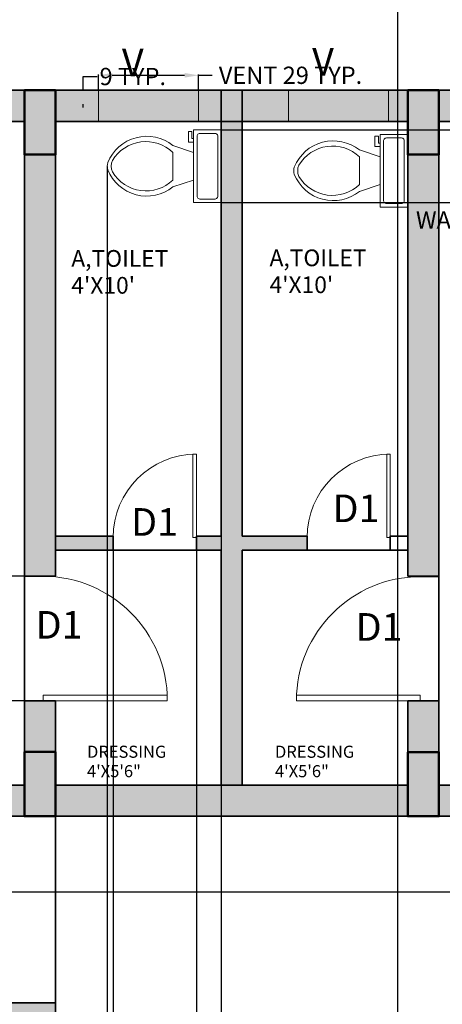
# Model space of a CAD drawing. Units: inches. Extents: x 460 to 1030, y -658 to 271.
# Tile 8 of 10: x 690 to 813, y -174 to 111. Entities that reach past the tile are written whole.
import ezdxf

# ---------------------------------------------------------------- set-up
doc = ezdxf.new("R2010")
doc.units = ezdxf.units.IN
doc.header["$MEASUREMENT"] = 0
for name, color, linetype, lineweight in [('A-ANNO-DIMS', 2, 'Continuous', 18), ('A-ANNO-TEXT', 7, 'Continuous', 18), ('A-AREA-IDEN', 7, 'Continuous', 25), ('A-COLS', 7, 'Continuous', 50), ('A-DOOR', 3, 'Continuous', 20), ('A-FLOR-FIXT', 9, 'Continuous', 18), ('A-GLAZ', 4, 'Continuous', 20), ('A-GLAZ-PATT', 4, 'Continuous', 13), ('A-WALL', 7, 'Continuous', 35), ('A-WALL-PATT', 5, 'Continuous', 13)]:
    doc.layers.add(name, color=color, linetype=linetype, lineweight=lineweight)
doc.layers.add('A-COLS-PATT', color=7, linetype='Continuous', lineweight=13, true_color=0xffffff)
doc.styles.get("Standard").update_dxf_attribs({"font": 'arial.ttf'})
doc.dimstyles.get("Standard").update_dxf_attribs({"dimtxt": 5, "dimasz": 4, "dimexe": 0.18, "dimexo": 0.0625, "dimgap": 0.09, "dimtad": 0, "dimtih": 1, "dimtoh": 1, "dimdec": 1, "dimzin": 0, "dimdsep": 46, "dimlunit": 4, "dimtxsty": 'Standard', "dimcen": 0.09, "dimadec": 0, "dimazin": 0, "dimtfac": 1, "dimtdec": 1, "dimtofl": 0, "dimtmove": 0, "dimatfit": 3, "dimfxl": 1, "dimtolj": 1, "dimtzin": 0, "dimarcsym": 0})

# ---------------------------------------------------------------- blocks, each defined once
blk = doc.blocks.new('*U2')
for p, q in [((0, 0), (0, -6)), ((40, 0), (40, -6))]:
    blk.add_line(p, q)
blk.add_lwpolyline([(0, 0), (0, 40), (1.75, 40), (1.75, 0)], close=True)
blk.add_arc((0, 0), 40, 0, 90)
blk = doc.blocks.new('*U4')
for p, q in [((9.5, -6), (9.5, -2)), ((-10, -8.5), (-8, -8.5)), ((-10, -9.5), (-10, -8.5)), ((-8, -8.5), (-8, -8)), ((-7, -8), (-7, -9.5)), ((-4, -8), (-6, -14)), ((4, -8), (6, -14)), ((-7, -9.5), (-10, -9.5)), ((4, -14), (-4, -14))]:
    blk.add_line(p, q)
blk.add_lwpolyline([(10.5, -8), (10.5, 0), (-10.5, 0), (-10.5, -8)], close=True)
for points in [[(-9.5, -2), (-9.5, -6)], [(8.5, -1), (-8.5, -1)], [(-8.5, -7), (8.5, -7)]]:
    blk.add_lwpolyline(points)
for centre, radius, start, end in [((-8.62, -1.88), 0.884, 81.8699, 188.1301), ((8.62, -1.88), 0.884, 351.8699, 98.1301), ((-8.62, -6.12), 0.884, 171.8699, 278.1301), ((8.62, -6.12), 0.884, 261.8699, 8.1301), ((3.52, -21.58), 12.17, 141.4691, 247.9714), ((4.2, -21.82), 11.33, 136.3677, 238.9468), ((-3.52, -21.58), 12.17, 292.0284, 38.5307), ((-4.2, -21.82), 11.33, 301.053, 43.6321), ((0, -27.88), 4, 245.7318, 294.2682), ((0, -29), 4, 254.8605, 285.1395)]:
    blk.add_arc(centre, radius, start, end)
blk = doc.blocks.new('COL-RECT-TYPE-A')
blk.add_lwpolyline([(0, 0), (9, 0), (9, -18.58), (0, -18.58)], close=True)
blk = doc.blocks.new('VENT-TOILET')
blk.add_lwpolyline([(0, 0), (-28.98, 0), (-28.98, 9), (0, 9)], close=True)
blk = doc.blocks.new('*D27')
at = {"layer": 'A-ANNO-DIMS', "color": 0, "lineweight": -2, "transparency": 16777216}
for p, q in [((827.46, 81.27), (836.13, 81.27)), ((835.95, 77.27), (835.95, 55.44)), ((835.95, 28.26), (835.95, 50.09)), ((827.46, 24.26), (836.13, 24.26))]:
    blk.add_line(p, q, dxfattribs=at)
at = {"layer": 'A-ANNO-DIMS', "color": 0, "transparency": 16777216}
for points in [[(835.28, 77.27), (836.62, 77.27), (835.95, 81.27)], [(835.28, 28.26), (836.62, 28.26), (835.95, 24.26)]]:
    blk.add_solid(points, dxfattribs=at)
at = {"layer": 'Defpoints', "color": 0, "transparency": 16777216}
for p in [(827.4, 81.27), (827.4, 24.26), (835.95, 24.26)]:
    blk.add_point(p, dxfattribs=at)
at = {"layer": 'A-ANNO-DIMS', "color": 0, "transparency": 16777216, "insert": (835.95, 52.77), "char_height": 5, "attachment_point": 5}
blk.add_mtext('\\A1;WARDROBE 57 TYP.', dxfattribs=at)
blk = doc.blocks.new('*D29')
at = {"layer": 'A-ANNO-DIMS', "color": 0, "lineweight": -2, "transparency": 16777216}
for p, q in [((713.2, 90.34), (713.2, 94.8)), ((717.2, 94.62), (738.18, 94.62)), ((742.18, 90.34), (742.18, 94.8)), ((742.18, 94.62), (746.18, 94.62))]:
    blk.add_line(p, q, dxfattribs=at)
at = {"layer": 'A-ANNO-DIMS', "color": 0, "transparency": 16777216}
for points in [[(717.2, 95.29), (717.2, 93.95), (713.2, 94.62)], [(738.18, 95.29), (738.18, 93.95), (742.18, 94.62)]]:
    blk.add_solid(points, dxfattribs=at)
at = {"layer": 'Defpoints', "color": 0, "transparency": 16777216}
for p in [(742.18, 94.62), (713.2, 90.27), (742.18, 90.27)]:
    blk.add_point(p, dxfattribs=at)
at = {"layer": 'A-ANNO-DIMS', "color": 0, "transparency": 16777216, "insert": (768.85, 94.62), "char_height": 5, "attachment_point": 5}
blk.add_mtext('\\A1;VENT 29 TYP.', dxfattribs=at)
blk = doc.blocks.new('*D30')
at = {"layer": 'A-ANNO-DIMS', "color": 0, "lineweight": -2, "transparency": 16777216}
for p, q in [((708.85, 90.27), (708.85, 94.27)), ((708.85, 94.27), (712.85, 94.27)), ((713.14, 90.27), (708.67, 90.27)), ((708.85, 85.27), (708.85, 86.27)), ((713.14, 81.27), (708.67, 81.27))]:
    blk.add_line(p, q, dxfattribs=at)
at = {"layer": 'A-ANNO-DIMS', "color": 0, "transparency": 16777216}
for points in [[(708.19, 86.27), (709.52, 86.27), (708.85, 90.27)], [(708.19, 85.27), (709.52, 85.27), (708.85, 81.27)]]:
    blk.add_solid(points, dxfattribs=at)
at = {"layer": 'Defpoints', "color": 0, "transparency": 16777216}
for p in [(708.85, 90.27), (713.2, 90.27), (713.2, 81.27)]:
    blk.add_point(p, dxfattribs=at)
at = {"layer": 'A-ANNO-DIMS', "color": 0, "transparency": 16777216, "insert": (723.17, 94.27), "char_height": 5, "attachment_point": 5}
blk.add_mtext('\\A1;9 TYP.', dxfattribs=at)
blk = doc.blocks.new('*D43')
at = {"layer": 'A-ANNO-DIMS', "color": 0, "lineweight": -2, "transparency": 16777216}
for p, q in [((562.8, 90.34), (562.8, 267.89)), ((940.8, 90.34), (940.8, 267.89)), ((566.8, 267.71), (746.18, 267.71)), ((936.8, 267.71), (757.41, 267.71))]:
    blk.add_line(p, q, dxfattribs=at)
at = {"layer": 'A-ANNO-DIMS', "color": 0, "transparency": 16777216}
for points in [[(566.8, 268.38), (566.8, 267.04), (562.8, 267.71)], [(936.8, 268.38), (936.8, 267.04), (940.8, 267.71)]]:
    blk.add_solid(points, dxfattribs=at)
at = {"layer": 'Defpoints', "color": 0, "transparency": 16777216}
for p in [(940.8, 267.71), (562.8, 90.27), (940.8, 90.27)]:
    blk.add_point(p, dxfattribs=at)
at = {"layer": 'A-ANNO-DIMS', "color": 0, "transparency": 16777216, "insert": (751.8, 267.71), "char_height": 5, "attachment_point": 5}
blk.add_mtext('\\A1;378', dxfattribs=at)
blk = doc.blocks.new('*D48')
at = {"layer": 'A-ANNO-DIMS', "color": 0, "lineweight": -2, "transparency": 16777216}
for p, q in [((799.88, -611.66), (799.88, 267.89)), ((941.7, -611.66), (941.7, 267.89)), ((803.88, 267.71), (860.58, 267.71)), ((937.7, 267.71), (881, 267.71))]:
    blk.add_line(p, q, dxfattribs=at)
at = {"layer": 'A-ANNO-DIMS', "color": 0, "transparency": 16777216}
for points in [[(803.88, 268.38), (803.88, 267.04), (799.88, 267.71)], [(937.7, 268.38), (937.7, 267.04), (941.7, 267.71)]]:
    blk.add_solid(points, dxfattribs=at)
at = {"layer": 'Defpoints', "color": 0, "transparency": 16777216}
for p in [(941.7, 267.71), (799.88, -611.73), (941.7, -611.73)]:
    blk.add_point(p, dxfattribs=at)
at = {"layer": 'A-ANNO-DIMS', "color": 0, "transparency": 16777216, "insert": (870.79, 267.71), "char_height": 5, "attachment_point": 5}
blk.add_mtext('\\A1;141.82', dxfattribs=at)
blk = doc.blocks.new('*D55')
at = {"layer": 'A-ANNO-DIMS', "color": 0, "lineweight": -2, "transparency": 16777216}
for p, q in [((894.56, -119.73), (470.68, -119.73)), ((470.86, -123.73), (470.86, -128.08)), ((470.86, -137.72), (470.86, -133.37)), ((894.55, -141.72), (470.68, -141.72))]:
    blk.add_line(p, q, dxfattribs=at)
at = {"layer": 'A-ANNO-DIMS', "color": 0, "transparency": 16777216}
for points in [[(470.19, -123.73), (471.52, -123.73), (470.86, -119.73)], [(470.19, -137.72), (471.52, -137.72), (470.86, -141.72)]]:
    blk.add_solid(points, dxfattribs=at)
at = {"layer": 'Defpoints', "color": 0, "transparency": 16777216}
for p in [(470.86, -119.73), (894.62, -119.73), (894.61, -141.72)]:
    blk.add_point(p, dxfattribs=at)
at = {"layer": 'A-ANNO-DIMS', "color": 0, "transparency": 16777216, "insert": (470.86, -130.72), "char_height": 5, "attachment_point": 5}
blk.add_mtext('\\A1;21.995', dxfattribs=at)
blk = doc.blocks.new('*D57')
at = {"layer": 'A-ANNO-DIMS', "color": 0, "lineweight": -2, "transparency": 16777216}
for p, q in [((717.53, -38.79), (717.53, -654.61)), ((741.59, -38.79), (741.59, -654.61)), ((713.53, -654.43), (709.53, -654.43)), ((745.59, -654.43), (749.59, -654.43))]:
    blk.add_line(p, q, dxfattribs=at)
at = {"layer": 'A-ANNO-DIMS', "color": 0, "transparency": 16777216}
for points in [[(713.53, -653.77), (713.53, -655.1), (717.53, -654.43)], [(745.59, -653.77), (745.59, -655.1), (741.59, -654.43)]]:
    blk.add_solid(points, dxfattribs=at)
at = {"layer": 'Defpoints', "color": 0, "transparency": 16777216}
for p in [(717.53, -38.73), (741.59, -38.73), (741.59, -654.43)]:
    blk.add_point(p, dxfattribs=at)
at = {"layer": 'A-ANNO-DIMS', "color": 0, "transparency": 16777216, "insert": (729.56, -654.43), "char_height": 5, "attachment_point": 5}
blk.add_mtext('\\A1;24.065', dxfattribs=at)
blk = doc.blocks.new('*D58')
at = {"layer": 'A-ANNO-DIMS', "color": 0, "lineweight": -2, "transparency": 16777216}
for p, q in [((691.73, -50.3), (470.68, -50.3)), ((470.86, -54.3), (470.86, -65.65)), ((470.86, -82.3), (470.86, -70.94)), ((691.73, -86.3), (470.68, -86.3))]:
    blk.add_line(p, q, dxfattribs=at)
at = {"layer": 'A-ANNO-DIMS', "color": 0, "transparency": 16777216}
for points in [[(470.19, -54.3), (471.52, -54.3), (470.86, -50.3)], [(470.19, -82.3), (471.52, -82.3), (470.86, -86.3)]]:
    blk.add_solid(points, dxfattribs=at)
at = {"layer": 'Defpoints', "color": 0, "transparency": 16777216}
for p in [(691.8, -50.3), (470.86, -86.3), (691.8, -86.3)]:
    blk.add_point(p, dxfattribs=at)
at = {"layer": 'A-ANNO-DIMS', "color": 0, "transparency": 16777216, "insert": (470.86, -68.3), "char_height": 5, "attachment_point": 5}
blk.add_mtext('\\A1;36', dxfattribs=at)
blk = doc.blocks.new('*D72')
at = {"layer": 'A-ANNO-DIMS', "color": 0, "lineweight": -2, "transparency": 16777216}
for p, q in [((715.8, 68.25), (715.8, -654.61)), ((748.8, 57.75), (748.8, -654.61)), ((719.8, -654.43), (728.63, -654.43)), ((744.8, -654.43), (735.97, -654.43))]:
    blk.add_line(p, q, dxfattribs=at)
at = {"layer": 'A-ANNO-DIMS', "color": 0, "transparency": 16777216}
for points in [[(719.8, -653.77), (719.8, -655.1), (715.8, -654.43)], [(744.8, -653.77), (744.8, -655.1), (748.8, -654.43)]]:
    blk.add_solid(points, dxfattribs=at)
at = {"layer": 'Defpoints', "color": 0, "transparency": 16777216}
for p in [(715.8, 68.31), (748.8, 57.81), (748.8, -654.43)]:
    blk.add_point(p, dxfattribs=at)
at = {"layer": 'A-ANNO-DIMS', "color": 0, "transparency": 16777216, "insert": (732.3, -654.43), "char_height": 5, "attachment_point": 5}
blk.add_mtext('\\A1;33', dxfattribs=at)
blk = doc.blocks.new('*D73')
at = {"layer": 'A-ANNO-DIMS', "color": 0, "lineweight": -2, "transparency": 16777216}
for p, q in [((748.86, 78.81), (1022.03, 78.81)), ((1021.85, 74.81), (1021.85, 70.92)), ((1021.85, 61.81), (1021.85, 65.71)), ((748.86, 57.81), (1022.03, 57.81))]:
    blk.add_line(p, q, dxfattribs=at)
at = {"layer": 'A-ANNO-DIMS', "color": 0, "transparency": 16777216}
for points in [[(1021.18, 74.81), (1022.51, 74.81), (1021.85, 78.81)], [(1021.18, 61.81), (1022.51, 61.81), (1021.85, 57.81)]]:
    blk.add_solid(points, dxfattribs=at)
at = {"layer": 'Defpoints', "color": 0, "transparency": 16777216}
for p in [(748.8, 78.81), (748.8, 57.81), (1021.85, 57.81)]:
    blk.add_point(p, dxfattribs=at)
at = {"layer": 'A-ANNO-DIMS', "color": 0, "transparency": 16777216, "insert": (1021.85, 68.31), "char_height": 5, "attachment_point": 5}
blk.add_mtext('\\A1;21', dxfattribs=at)

msp = doc.modelspace()

# ---------------------------------------------------------------- hatches: boundary and pattern name
at = {"layer": 'A-COLS-PATT'}
h = msp.add_hatch(color=256, dxfattribs=at)
h.dxf.hatch_style = 1
h.paths.add_polyline_path([(571.7961, 90.2738), (562.7961, 90.2738), (562.7961, 71.6966), (571.7961, 71.6966)])
h.paths.add_polyline_path([(700.7961, 90.2738), (691.7961, 90.2738), (691.7961, 71.6966), (700.7961, 71.6966)])
h.paths.add_polyline_path([(811.7961, 90.2738), (802.7961, 90.2738), (802.7961, 71.6966), (811.7961, 71.6966)])
h.paths.add_polyline_path([(940.7961, 90.2738), (931.7961, 90.2738), (931.7961, 71.6966), (940.7961, 71.6966)])
h.paths.add_polyline_path([(940.7961, -101.149), (931.7961, -101.149), (931.7961, -119.7262), (940.7961, -119.7262)])
h.paths.add_polyline_path([(940.7961, -268.3723), (931.7961, -268.3723), (931.7961, -287.7262), (940.7961, -287.7262)])
h.paths.add_polyline_path([(803.0275, -281.7262), (789.8237, -281.7262), (789.8237, -287.7262), (803.0275, -287.7262)])
h.paths.add_polyline_path([(700.7961, -303.809), (691.7961, -303.809), (691.7961, -323.8443), (700.7961, -323.8443)])
h.paths.add_polyline_path([(571.7961, -303.809), (562.7961, -303.809), (562.7961, -323.8443), (571.7961, -323.8443)])
h.paths.add_polyline_path([(571.7961, -413.1453), (562.7961, -413.1453), (562.7961, -432.4659), (571.7961, -432.4659)])
h.paths.add_polyline_path([(571.7961, -101.149), (562.7961, -101.149), (562.7961, -119.7262), (571.7961, -119.7262)])
h.paths.add_polyline_path([(700.7961, -101.0985), (691.7961, -101.0985), (691.7961, -119.7262), (700.7961, -119.7262)])
h.paths.add_polyline_path([(811.7961, -101.149), (802.7961, -101.149), (802.7961, -119.7262), (811.7961, -119.7262)])
at = {"layer": 'A-GLAZ-PATT'}
h = msp.add_hatch(color=256, dxfattribs=at)
h.dxf.hatch_style = 1
h.paths.add_polyline_path([(571.7961, -343.9041), (562.7961, -343.9041), (562.7961, -384.3969), (571.7961, -384.3969)])
h.paths.add_polyline_path([(571.7961, -143.2895), (562.7961, -143.2895), (562.7961, -168.3798), (571.7961, -168.3798)])
h.paths.add_polyline_path([(571.7961, -49.2966), (562.7961, -49.2966), (562.7961, -90.3192), (571.7961, -90.3192)])
h.paths.add_polyline_path([(666.4584, 90.2738), (634.2742, 90.2738), (634.2742, 81.2738), (666.4584, 81.2738)])
h.paths.add_polyline_path([(742.1779, 90.2738), (713.201, 90.2738), (713.201, 81.2738), (742.1779, 81.2738)])
h.paths.add_polyline_path([(797.2395, 90.2738), (768.2626, 90.2738), (768.2626, 81.2738), (797.2395, 81.2738)])
h.paths.add_polyline_path([(918.7723, 90.2738), (881.2728, 90.2738), (881.2728, 81.2738), (918.7723, 81.2738)])
h.paths.add_polyline_path([(940.7961, -60.0042), (931.7961, -60.0042), (931.7961, -95.7262), (940.7961, -95.7262)])
h.paths.add_polyline_path([(940.7961, -163.6558), (931.7961, -163.6558), (931.7961, -230.2946), (940.7961, -230.2946)])
h.paths.add_polyline_path([(913.7961, -331.7262), (835.7961, -331.7262), (835.7961, -332.7262), (913.7961, -332.7262)])
h.paths.add_polyline_path([(871.4559, -281.7262), (831.4302, -281.7262), (831.4302, -287.7262), (871.4559, -287.7262)])
h.paths.add_polyline_path([(774.8576, -281.7262), (716.7073, -281.7262), (716.7073, -287.7262), (774.8576, -287.7262)])
at = {"layer": 'A-WALL-PATT'}
h = msp.add_hatch(color=256, dxfattribs=at)
h.dxf.hatch_style = 1
h.paths.add_polyline_path([(634.2742, 90.2738), (571.7961, 90.2738), (571.7961, 81.2738), (634.2742, 81.2738)])
h.paths.add_polyline_path([(691.7961, 90.2738), (666.4584, 90.2738), (666.4584, 81.2738), (691.7961, 81.2738)])
h.paths.add_polyline_path([(713.201, 90.2738), (700.7961, 90.2738), (700.7961, 81.2738), (713.201, 81.2738)])
h.paths.add_polyline_path([(748.7961, 90.2738), (742.1779, 90.2738), (742.1779, 81.2738), (748.7961, 81.2738)])
h.paths.add_polyline_path([(768.2626, 90.2738), (754.7961, 90.2738), (754.7961, 81.2738), (768.2626, 81.2738)])
h.paths.add_polyline_path([(802.7961, 90.2738), (797.2395, 90.2738), (797.2395, 81.2738), (802.7961, 81.2738)])
h.paths.add_polyline_path([(881.2728, 90.2738), (811.7961, 90.2738), (811.7961, 81.2738), (881.2728, 81.2738)])
h.paths.add_polyline_path([(931.7961, 90.2738), (918.7723, 90.2738), (918.7723, 81.2738), (931.7961, 81.2738)])
h.paths.add_polyline_path([(940.7961, 71.6966), (931.7961, 71.6966), (931.7961, -60.0042), (940.7961, -60.0042)])
h.paths.add_polyline_path([(940.7961, -95.7262), (931.7961, -95.7262), (931.7961, -101.149), (940.7961, -101.149)])
h.paths.add_polyline_path([(931.7961, -110.7262), (894.6225, -110.7262), (894.6225, -119.7262), (931.7961, -119.7262)])
h.paths.add_polyline_path([(858.6225, -110.7262), (811.7961, -110.7262), (811.7961, -119.7262), (858.6225, -119.7262)])
h.paths.add_polyline_path([(940.7961, -119.7262), (931.7961, -119.7262), (931.7961, -141.7212), (931.7961, -163.6558), (940.7961, -163.6558)])
h.paths.add_polyline_path([(940.7961, -230.2946), (931.7961, -230.2946), (931.7961, -268.3723), (940.7961, -268.3723)])
h.paths.add_polyline_path([(931.7961, -281.7262), (908.3452, -281.7262), (908.3452, -285.0181), (908.3452, -287.7262), (931.7961, -287.7262)])
h.paths.add_polyline_path([(831.4302, -281.7262), (803.0275, -281.7262), (803.0275, -287.7262), (808.7961, -287.7262), (808.7961, -339.7262), (811.7961, -339.7262), (811.7961, -287.7262), (831.4302, -287.7262)])
h.paths.add_polyline_path([(789.8237, -281.7262), (774.8576, -281.7262), (774.8576, -287.7262), (789.8237, -287.7262)])
h.paths.add_polyline_path([(716.7073, -281.7262), (700.7961, -281.7262), (700.7961, -271.1977), (691.7961, -271.1977), (691.7961, -281.7262), (682.4735, -281.7262), (682.4735, -287.7262), (691.7961, -287.7262), (691.7961, -303.809), (700.7961, -303.809), (700.7961, -287.7262), (716.7073, -287.7262)])
h.paths.add_polyline_path([(700.7961, -323.8443), (691.7961, -323.8443), (691.7961, -413.1453), (700.7961, -413.1453)])
h.paths.add_polyline_path([(940.7961, -287.7262), (937.7961, -287.7262), (937.7961, -339.7262), (940.7961, -339.7262)])
h.paths.add_polyline_path([(937.7961, -336.7262), (811.7961, -336.7262), (811.7961, -339.7262), (937.7961, -339.7262)])
h.paths.add_polyline_path([(835.7961, -329.7262), (811.7961, -329.7262), (811.7961, -332.7262), (835.7961, -332.7262)])
h.paths.add_polyline_path([(937.7961, -329.7262), (913.7961, -329.7262), (913.7961, -332.7262), (937.7961, -332.7262)])
h.paths.add_polyline_path([(691.7961, -419.7262), (681.4044, -419.7262), (681.4044, -428.7262), (691.7961, -428.7262)])
h.paths.add_polyline_path([(691.7961, -476.7262), (571.7961, -476.7262), (571.7961, -485.7262), (691.7961, -485.7262)])
h.paths.add_polyline_path([(571.7961, -465.0348), (568.223, -465.0348), (562.7961, -465.0348), (562.7961, -476.7262), (571.7961, -476.7262)])
h.paths.add_polyline_path([(571.7961, -432.4659), (562.7961, -432.4659), (562.7961, -441.1912), (571.7961, -441.1912)])
h.paths.add_polyline_path([(571.7961, -384.3969), (562.7961, -384.3969), (562.7961, -413.1453), (571.7961, -413.1453)])
h.paths.add_polyline_path([(571.7961, -323.8443), (562.7961, -323.8443), (562.7961, -343.9041), (571.7961, -343.9041)])
h.paths.add_polyline_path([(571.7961, -287.7262), (646.4735, -287.7262), (646.4735, -281.7262), (571.7961, -281.7262), (571.7961, -258.1542), (571.7961, -233.7262), (566.4164, -233.7262), (562.7961, -233.7262), (562.7961, -303.809), (571.7961, -303.809)])
h.paths.add_polyline_path([(571.7961, -179.7262), (691.7961, -179.7262), (691.7961, -197.5753), (700.7961, -197.5753), (700.7961, -173.7262), (647.7961, -173.7262), (647.7961, -165.5723), (643.7961, -165.5723), (643.7961, -173.7262), (571.7961, -173.7262), (571.7961, -168.3798), (562.7961, -168.3798), (562.7961, -197.7262), (571.7961, -197.7262)])
h.paths.add_polyline_path([(647.7961, -110.7262), (571.7961, -110.7262), (571.7961, -119.7262), (643.7961, -119.7262), (643.7961, -141.5723), (647.7961, -141.5723)])
h.paths.add_polyline_path([(691.7961, -110.7262), (683.7961, -110.7262), (683.7961, -114.3453), (683.7961, -119.7262), (691.7961, -119.7262)])
h.paths.add_polyline_path([(571.7961, -119.7262), (562.7961, -119.7262), (562.7961, -143.2895), (571.7961, -143.2895)])
h.paths.add_polyline_path([(571.7961, -90.3192), (562.7961, -90.3192), (562.7961, -101.149), (571.7961, -101.149)])
h.paths.add_polyline_path([(571.7961, 71.6966), (562.7961, 71.6966), (562.7961, -49.2966), (571.7961, -49.2966)])
h.paths.add_polyline_path([(700.7961, 71.6966), (691.7961, 71.6966), (691.7961, -50.298), (700.7961, -50.298)])
h.paths.add_polyline_path([(754.7961, 81.2738), (748.7961, 81.2738), (748.7961, -38.7262), (741.5908, -38.7262), (741.5908, -39.109), (741.5908, -42.7262), (748.7961, -42.7262), (748.7961, -110.7262), (754.7961, -110.7262), (754.7961, -42.7262), (773.6274, -42.7262), (773.6274, -38.7262), (754.7961, -38.7262)])
h.paths.add_polyline_path([(717.4759, -38.7262), (700.7961, -38.7262), (700.7961, -42.7262), (717.4759, -42.7262)])
h.paths.add_polyline_path([(811.7961, 71.6966), (802.7961, 71.6966), (802.7961, -50.298), (811.7961, -50.298)])
h.paths.add_polyline_path([(811.7961, -86.298), (806.4164, -86.298), (802.7961, -86.298), (802.7961, -101.149), (811.7961, -101.149)])
h = msp.add_hatch(color=256, dxfattribs=at)
h.dxf.hatch_style = 1
h.paths.add_polyline_path([(700.7961, -86.298), (697.1925, -86.298), (691.7961, -86.298), (691.7961, -101.0985), (700.7961, -101.0985)])
h.paths.add_polyline_path([(802.7961, -110.7262), (700.7961, -110.7262), (700.7961, -119.7262), (802.7961, -119.7262)])
h.paths.add_polyline_path([(754.7961, 90.2738), (748.7961, 90.2738), (748.7961, 81.2738), (754.7961, 81.2738)])

# ---------------------------------------------------------------- linework, layer by layer
at = {"layer": 'A-COLS'}
msp.add_lwpolyline([(700.7961, -119.7262), (691.7961, -119.7262), (691.7961, -101.0985), (700.7961, -101.0985)], close=True, dxfattribs=at)
at = {"layer": 'A-WALL'}
for p, q in [((940.7961, 90.2738), (562.7961, 90.2738)), ((691.7961, 90.2738), (691.7961, -119.7262)), ((700.7961, 90.2738), (700.7961, -50.298)), ((748.7961, 90.2738), (748.7961, -38.7262)), ((754.7961, 90.2738), (754.7961, -38.7262)), ((802.7961, 90.2738), (802.7961, -50.298)), ((811.7961, 90.2738), (811.7961, -119.7262)), ((691.7961, 81.2738), (571.7961, 81.2738)), ((802.7961, 81.2738), (700.7961, 81.2738)), ((748.7961, 81.2738), (748.7961, -38.7262)), ((754.7961, 81.2738), (754.7961, -38.7262)), ((931.7961, 81.2738), (811.7961, 81.2738)), ((717.5258, -38.7262), (700.7961, -38.7262)), ((717.5258, -38.7262), (717.5258, -42.7262)), ((748.7961, -38.7262), (741.5908, -38.7262)), ((741.5908, -42.7262), (741.5908, -38.7262)), ((773.6773, -38.7262), (754.7961, -38.7262)), ((773.6773, -38.7262), (773.6773, -42.7262)), ((802.7961, -38.7262), (797.7423, -38.7262)), ((797.7423, -42.7262), (797.7423, -38.7262)), ((748.7961, -42.7262), (700.7961, -42.7262)), ((748.7961, -42.7262), (748.7961, -110.7262)), ((802.7961, -42.7262), (754.7961, -42.7262)), ((754.7961, -42.7262), (754.7961, -110.7262)), ((691.7961, -50.298), (700.7961, -50.298)), ((802.7961, -50.298), (811.7961, -50.298)), ((700.7961, -86.298), (691.7961, -86.298)), ((700.7961, -86.298), (700.7961, -281.7262)), ((811.7961, -86.298), (802.7961, -86.298)), ((802.7961, -86.298), (802.7961, -119.7262)), ((691.7961, -110.7262), (683.7961, -110.7262)), ((802.7961, -110.7262), (700.7961, -110.7262)), ((858.6225, -110.7262), (811.7961, -110.7262)), ((940.7961, -119.7262), (647.7961, -119.7262)), ((700.7961, -173.7262), (647.7961, -173.7262))]:
    msp.add_line(p, q, dxfattribs=at)

# ---------------------------------------------------------------- block references
at = {"layer": 'A-COLS'}
for p in [(691.7961, 90.2738), (802.7961, 90.2738), (802.7961, -101.149)]:
    msp.add_blockref('COL-RECT-TYPE-A', p, dxfattribs=at)
at = {"layer": 'A-DOOR', "xscale": -0.6028704174083245, "yscale": 0.6028704174083245, "zscale": 0.6028704174083245}
for p in [(741.5908, -39.109), (797.7423, -39.109)]:
    msp.add_blockref('*U2', p, dxfattribs=at)
at = {"layer": 'A-DOOR'}
for p, xscale, yscale, zscale, rotation in [((697.1925, -86.298), -0.8994006151666546, 0.8994006151666546, 0.8994006151666546, 270), ((806.4164, -86.298), 0.8966154602300187, 0.8966154602300187, 0.8966154602300187, 90.00000000000003)]:
    msp.add_blockref('*U2', p, dxfattribs=dict(at, xscale=xscale, yscale=yscale, zscale=zscale, rotation=rotation))
at = {"layer": 'A-FLOR-FIXT', "rotation": 270}
for p in [(748.7961, 68.3148), (802.7961, 67.0102)]:
    msp.add_blockref('*U4', p, dxfattribs=at)
at = {"layer": 'A-GLAZ'}
for p in [(742.1779, 81.2738), (797.2395, 81.2738)]:
    msp.add_blockref('VENT-TOILET', p, dxfattribs=at)

# ---------------------------------------------------------------- texts
at = {"layer": 'A-ANNO-TEXT'}
for s, p in [('V', (775.108, 94.542)), ('V', (720.0333, 94.309)), ('D1', (781.0275, -34.6506)), ('D1', (722.6977, -38.5975)), ('D1', (695.0518, -68.3511)), ('D1', (787.7111, -68.9584))]:
    msp.add_text(s, height=8, dxfattribs=at).set_placement(p)
at = {"layer": 'A-AREA-IDEN'}
for s, height, p in [('A,TOILET', 4.84251, (705.3679, 39.2224)), ('A,TOILET', 4.84251, (762.7636, 39.3883)), ("4'X10'", 4.84251, (705.3679, 31.4433)), ("4'X10'", 4.84251, (762.7636, 31.6092)), ('DRESSING ', 3.49872, (709.9158, -102.809)), ('DRESSING ', 3.49872, (764.3402, -102.809)), ('4\'X5\'6"', 3.49872, (709.9158, -108.4294)), ('4\'X5\'6"', 3.49872, (764.3402, -108.4294))]:
    msp.add_text(s, height=height, dxfattribs=at).set_placement(p)

# ---------------------------------------------------------------- dimensions: what is measured, and where the dimension line sits
at = {"layer": 'A-ANNO-DIMS'}
for base, p1, p2, override, picture, middle in [((940.7961, 267.7108), (562.7961, 90.2738), (940.7961, 90.2738), {"dimdec": 0, "dimlfac": 1, "dimrnd": 0, "dimzin": 0, "dimdsep": 46, "dimlunit": 2}, '*D43', (751.7961, 267.7108)), ((941.6978, 267.7108), (799.8801, -611.7262), (941.6978, -611.7262), {"dimdec": 2, "dimlfac": 1, "dimrnd": 0, "dimzin": 0, "dimdsep": 46, "dimlunit": 2}, '*D48', (870.7889, 267.7108)), ((748.7961, -654.4339), (715.7961, 68.3148), (748.7961, 57.8148), {"dimdec": 0, "dimlfac": 1, "dimrnd": 0, "dimzin": 0, "dimdsep": 46, "dimlunit": 2}, '*D72', (732.2961, -654.4339)), ((741.5908, -654.4339), (717.5258, -38.7262), (741.5908, -38.7262), {"dimdec": 3, "dimlfac": 1, "dimrnd": 0, "dimzin": 0, "dimdsep": 46, "dimlunit": 2}, '*D57', (729.5583, -654.4339))]:
    dim = msp.add_linear_dim(base=base, p1=p1, p2=p2, dimstyle='Standard', override=override, dxfattribs=at)
    dim.commit()
    dim.dimension.update_dxf_attribs({"geometry": picture, "text_midpoint": middle})
dim = msp.add_linear_dim(base=(742.1779, 94.6203), p1=(713.201, 90.2738), p2=(742.1779, 90.2738), text='VENT <> TYP.', dimstyle='Standard', override={"dimdec": 0, "dimlfac": 1, "dimrnd": 0, "dimzin": 0, "dimdsep": 46, "dimlunit": 2}, dxfattribs=at)
dim.commit()
dim.dimension.update_dxf_attribs({"geometry": '*D29', "text_midpoint": (768.8514, 94.6203)})
for base, p1, p2, angle, text, picture, middle in [((708.8544, 90.2738), (713.201, 81.2738), (713.201, 90.2738), 90, '<> TYP.', '*D30', (723.1713, 94.2738)), ((835.9484, 24.2594), (827.3963, 81.2738), (827.3963, 24.2594), 270, 'WARDROBE <> TYP.', '*D27', (835.9484, 52.7666))]:
    dim = msp.add_linear_dim(base=base, p1=p1, p2=p2, angle=angle, text=text, dimstyle='Standard', override={"dimdec": 0, "dimlfac": 1, "dimrnd": 0, "dimzin": 0, "dimdsep": 46, "dimlunit": 2}, dxfattribs=at)
    dim.commit()
    dim.dimension.update_dxf_attribs({"geometry": picture, "text_midpoint": middle})
for base, p1, p2, override, picture, middle in [((1021.8461, 57.8148), (748.7961, 78.8148), (748.7961, 57.8148), {"dimdec": 0, "dimlfac": 1, "dimrnd": 0, "dimzin": 0, "dimdsep": 46, "dimlunit": 2}, '*D73', (1021.8461, 68.3148)), ((470.8563, -86.298), (691.7961, -50.298), (691.7961, -86.298), {"dimdec": 0, "dimlfac": 1, "dimrnd": 0, "dimzin": 0, "dimdsep": 46, "dimlunit": 2}, '*D58', (470.8563, -68.298)), ((470.8563, -119.7262), (894.6132, -141.7212), (894.6225, -119.7262), {"dimdec": 3, "dimlfac": 1, "dimrnd": 0, "dimzin": 0, "dimdsep": 46, "dimlunit": 2}, '*D55', (470.8563, -130.7237))]:
    dim = msp.add_linear_dim(base=base, p1=p1, p2=p2, angle=90, dimstyle='Standard', override=override, dxfattribs=at)
    dim.commit()
    dim.dimension.update_dxf_attribs({"geometry": picture, "text_midpoint": middle})

doc.saveas('drawing.dxf')
